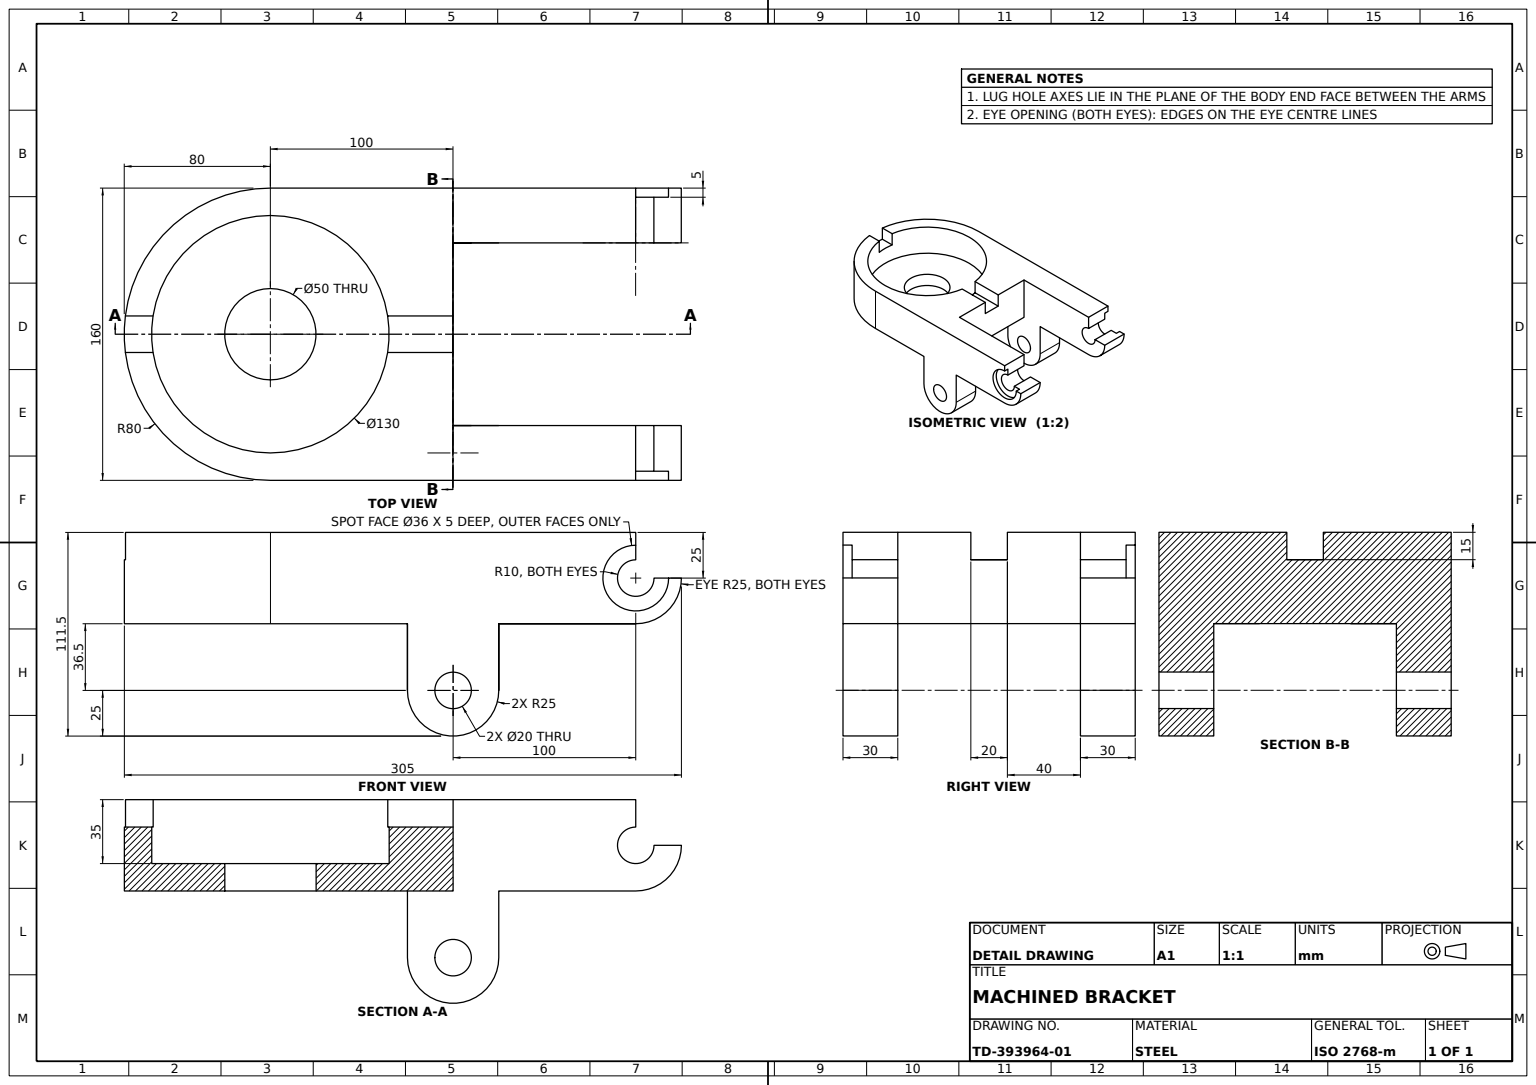
SolidWorks part; units mm, degrees
material "Plain Carbon Steel"
ref_plane "Front Plane" through (0, 0, 0) normal (0, 0, 1) x (1, 0, 0)
ref_plane "Top Plane" through (0, 0, 0) normal (0, 1, 0) x (1, 0, 0)
ref_plane "Right Plane" through (0, 0, 0) normal (1, 0, 0) x (0, 0, -1)
sketch "Base Plate Sketch" plane through (0, 0, 0) normal (0, 1, 0) x (1, 0, 0)
  line L0 (-79.3725, 10) -> (-64.2262, 10)
  line L6 (-64.2262, -10) -> (-79.3725, -10)
  line L7 (0, -80) -> (200, -80)
  line L8 (0, 80) -> (200, 80)
  line L9 (200, 80) -> (200, 50)
  line L10 (200, 50) -> (100, 50)
  line L11 (100, 50) -> (100, 10)
  line L12 (100, -50) -> (200, -50)
  line L13 (200, -50) -> (200, -80)
  line L14 (100, -10) -> (100, -50)
  line L15 (64.2262, -10) -> (100, -10)
  line L16 (64.2262, 10) -> (100, 10)
  arc A0 (-64.2262, -10) -> (64.2262, -10) centre (0, 0) ccw
  arc A2 (-79.3725, -10) -> (79.3725, -10) centre (0, 0) ccw
  arc A3 (64.2262, 10) -> (-64.2262, 10) centre (0, 0) ccw
  arc A4 (79.3725, 10) -> (-79.3725, 10) centre (0, 0) ccw
  point P5 (0, 10)
  point P6 (-80, 0)
  point P7 (-80, 10)
  point P8 (0, -10)
  point P9 (-80, -10)
  point P19 (0, -10)
  point P21 (100, 0)
  point P23 (0, 10)
  dimension "D1" = 160
  dimension "D2" = 130
  dimension "D4" = 10
  dimension "D6" = 20
  dimension "D5" = 10
  dimension "D7" = 30
  dimension "D8" = 200
  dimension "D9" = 100
  dimension "D10" = 100
  dimension "D11" = 200
  dimension "D12" = 35.7738
  dimension "D14" = 10
  dimension "D13" = 35.7738
  dimension "D15" = 10
extrude "Base Plate" add sketch "Base Plate Sketch" along normal blind 15 contours A2 L15 A0 L6 | L16 A4 L0 A3 | A4 L16 L11 L10 L9 L8 | A2 L7 L13 L12 L14 L15
sketch "Circular Housing Sketch" plane through (0, 0, 0) normal (0, -1, 0) x (1, 0, 0)
  line L0 (0, 80) -> (200, 80)
  line L1 (200, 80) -> (200, 50)
  line L2 (200, 50) -> (100, 50)
  line L3 (100, 50) -> (100, -50)
  line L4 (100, -50) -> (200, -50)
  line L5 (200, -50) -> (200, -80)
  line L6 (200, -80) -> (0, -80)
  circle A0 centre (0, 0) radius 80
  circle A1 centre (0, 0) radius 65
  arc M1 (0, 80) -> (-79.3725, 10) centre (0, 0) ccw
  line M2 (-79.3725, 10) -> (-64.2262, 10)
  arc M3 (-64.2262, 10) -> (64.2262, 10) centre (0, 0) cw
  line M4 (64.2262, 10) -> (100, 10)
  line M5 (100, 10) -> (100, 50)
  line M6 (100, 50) -> (200, 50)
  line M7 (200, 50) -> (200, 80)
  line M8 (200, 80) -> (0, 80)
  dimension "D1" = 130
extrude "Circular Housing" add sketch "Circular Housing Sketch" along normal blind 35 contours A0 M4 M1 M2 M3 | A1 A0 M2 M4 | A0 M4 M5 M6 M7 M8 | A0 L6 L5 L4 L3 M4
sketch "Housing Extension Sketch" plane through (0, -35, 0) normal (0, -1, 0) x (1, 0, 0)
  circle A0 centre (0, 0) radius 65
  circle A1 centre (0, 0) radius 25
  dimension "D1" = 130
  dimension "D2" = 50
extrude "Housing Extension" add sketch "Housing Extension Sketch" against normal blind 15
sketch "Clevis Lug Block Sketch" plane through (0, 0, 80) normal (0, 0, 1) x (1, 0, 0)
  line L0 (0, -35) -> (0, 15) construction
  line L1 (200, -35) -> (0, -35) construction
  line L2 (75, -71.5) -> (75, -35)
  line L3 (75, -35) -> (125, -35)
  line L4 (125, -35) -> (125, -71.5)
  circle A0 centre (100, -71.5) radius 10
  circle A1 centre (100, -71.5) radius 25
  line M4 (0, -35) -> (200, -35)
  dimension "D1" = 50
  dimension "D2" = 20
  dimension "D3" = 100
  dimension "D4" = 36.5
extrude "Clevis Lug Block" add sketch "Clevis Lug Block Sketch" against normal blind 30 contours A1 L4 L2 M4 | A1 A0
sketch "Clevis Lug Extension Sketch" plane through (0, 0, -80) normal (0, 0, -1) x (-1, 0, 0)
  line L0 (-125, -71.5) -> (-125, -35)
  line L1 (-125, -35) -> (-75, -35)
  line L2 (-75, -35) -> (-75, -71.5)
  circle A0 centre (-100, -71.5) radius 10
  circle A1 centre (-100, -71.5) radius 25
  line M2 (-200, -35) -> (0, -35)
  dimension "D1" = 20
extrude "Clevis Lug Extension" add sketch "Clevis Lug Extension Sketch" against normal blind 30 contours A1 L2 L0 M2 | A1 A0
sketch "Pivot Lug Sketch" plane through (0, 0, 80) normal (0, 0, 1) x (1, 0, 0)
  line L0 (200, -35) -> (200, 15) construction
  circle A0 centre (200, -10) radius 25
extrude "Pivot Lugs" add sketch "Pivot Lug Sketch" against normal blind 30
sketch "Pivot Pin Hole Sketch" plane through (0, 0, 80) normal (0, 0, 1) x (1, 0, 0)
  circle A0 centre (200, -10) radius 10
  dimension "D1" = 20
extrude "Pivot Pin Hole Ø20" cut sketch "Pivot Pin Hole Sketch" against normal blind 200
sketch "Clevis Slot Sketch" plane through (0, 0, 80) normal (0, 0, 1) x (1, 0, 0)
  line L0 (200, 15) -> (200, -10)
  line L1 (200, -10) -> (225, -10)
  arc A0 (200, -35) -> (200, 15) centre (200, -10) ccw construction
  arc A1 (200, 15) -> (225, -10) centre (200, -10) cw
  dimension "D1" = 25
extrude "Clevis Slot 25" cut sketch "Clevis Slot Sketch" against normal blind 200
sketch "Spot Face A Sketch" plane through (0, 0, 80) normal (0, 0, 1) x (1, 0, 0)
  circle A0 centre (200, -10) radius 18
  dimension "D1" = 36
extrude "Spot Face A Ø36x5" cut sketch "Spot Face A Sketch" against normal blind 5
sketch "Lug Fill Sketch" plane through (0, 0, -80) normal (0, 0, -1) x (-1, 0, 0)
  line L0 (-210, -10) -> (-225, -10)
  line L1 (-200, -20) -> (-200, -35)
  arc A0 (-210, -10) -> (-200, -20) centre (-200, -10) ccw
  arc A1 (-225, -10) -> (-200, -35) centre (-200, -10) ccw construction
  arc A2 (-225, -10) -> (-200, -35) centre (-200, -10) ccw
  dimension "D1" = 25
extrude "Lug Fill Boss" add sketch "Lug Fill Sketch" against normal blind 30
sketch "Spot Face B Sketch" plane through (0, 0, -80) normal (0, 0, -1) x (-1, 0, 0)
  circle A0 centre (-200, -10) radius 18
  dimension "D1" = 36
extrude "Spot Face B Ø36x5" cut sketch "Spot Face B Sketch" against normal blind 5
